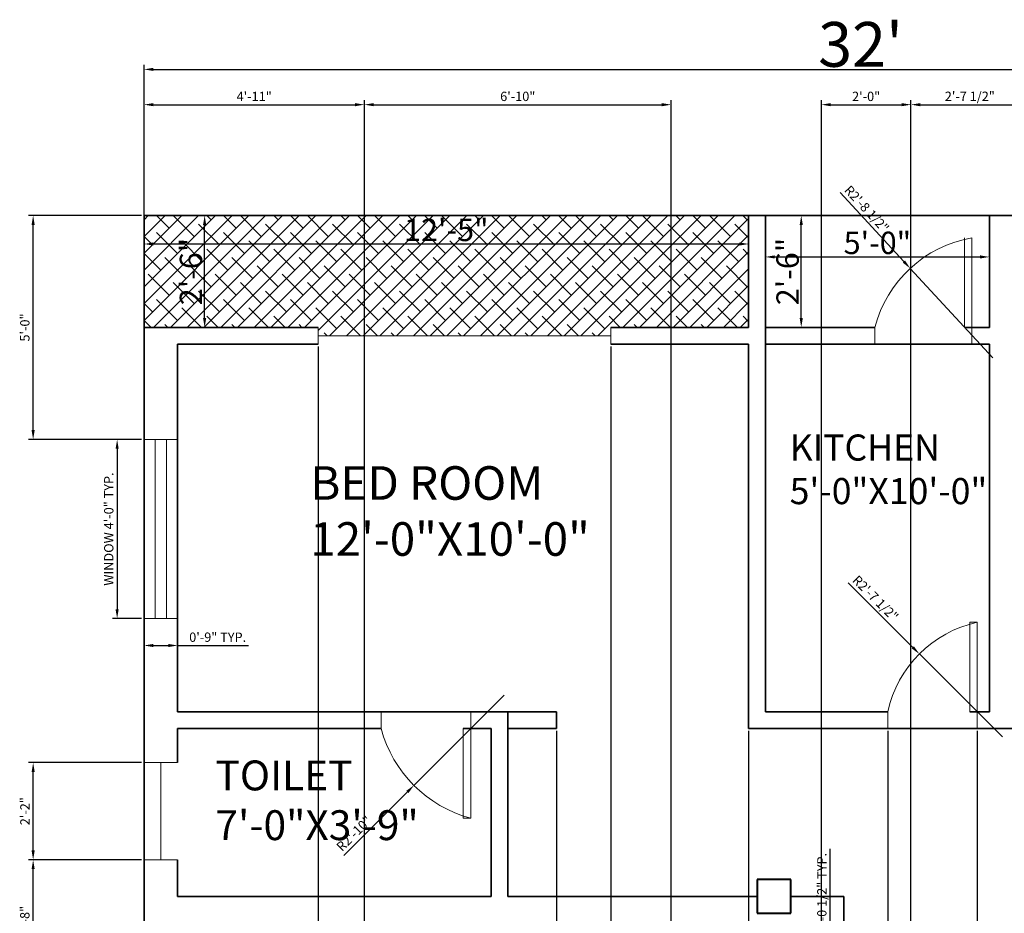
# Model space of a CAD drawing. Units: millimetres. Extents: x 2124 to 2653, y 1244 to 1836.
# Tile 3 of 4: x 2126 to 2390, y 1597 to 1836. Entities that reach past the tile are written whole.
import ezdxf

# ---------------------------------------------------------------- set-up
doc = ezdxf.new("R2010")
doc.units = ezdxf.units.MM
for name, color, linetype, lineweight in [('A-ANNO-DIMS', 2, 'Continuous', 18), ('A-AREA-IDEN', 7, 'Continuous', 18), ('A-COLS', 1, 'Continuous', 40), ('A-DOOR', 3, 'Continuous', 18), ('A-FLOR-PATT', 252, 'Continuous', 13), ('A-GLAZ', 4, 'Continuous', 18), ('A-WALL', 7, 'Continuous', 35)]:
    doc.layers.add(name, color=color, linetype=linetype, lineweight=lineweight)
doc.styles.get("Standard").update_dxf_attribs({"font": 'arial.ttf'})
doc.dimstyles.new('ISO-25', dxfattribs={"dimtxt": 2.5, "dimasz": 2.5, "dimexe": 1.25, "dimexo": 0.625, "dimtad": 1, "dimdec": 0, "dimlunit": 3, "dimtxsty": 'Standard', "dimcen": 2.5, "dimadec": 0, "dimazin": 0, "dimtfac": 1, "dimtdec": 0, "dimtmove": 0, "dimatfit": 3, "dimfxl": 1, "dimarcsym": 0})

# ---------------------------------------------------------------- blocks, each defined once
blk = doc.blocks.new('*D2')
at = {"layer": 'A-ANNO-DIMS', "color": 0, "lineweight": -2, "transparency": 16777216}
for p, q in [((2160.38, 1783.74), (2177.25, 1783.74)), ((2176, 1756.24), (2176, 1781.24)), ((2160.38, 1753.74), (2177.25, 1753.74))]:
    blk.add_line(p, q, dxfattribs=at)
at = {"layer": 'A-ANNO-DIMS', "color": 0, "transparency": 16777216}
for points in [[(2175.58, 1781.24), (2176.42, 1781.24), (2176, 1783.74)], [(2175.58, 1756.24), (2176.42, 1756.24), (2176, 1753.74)]]:
    blk.add_solid(points, dxfattribs=at)
at = {"layer": 'Defpoints', "color": 0, "transparency": 16777216}
for p in [(2159.76, 1783.74), (2176, 1783.74), (2159.76, 1753.74)]:
    blk.add_point(p, dxfattribs=at)
at = {"layer": 'A-ANNO-DIMS', "color": 0, "transparency": 16777216, "insert": (2172.34, 1768.74), "char_height": 2.5, "attachment_point": 5, "rotation": 90}
blk.add_mtext('{\\fCambria|b0|i0|c0|p18;\\H2.4x;2\'-6"}', dxfattribs=at)
blk = doc.blocks.new('*D3')
at = {"layer": 'A-ANNO-DIMS', "color": 0, "lineweight": -2, "transparency": 16777216}
for p, q in [((2326.88, 1783.74), (2337.1, 1783.74)), ((2335.85, 1756.24), (2335.85, 1781.24)), ((2326.88, 1753.74), (2337.1, 1753.74))]:
    blk.add_line(p, q, dxfattribs=at)
at = {"layer": 'A-ANNO-DIMS', "color": 0, "transparency": 16777216}
for points in [[(2335.44, 1781.24), (2336.27, 1781.24), (2335.85, 1783.74)], [(2335.44, 1756.24), (2336.27, 1756.24), (2335.85, 1753.74)]]:
    blk.add_solid(points, dxfattribs=at)
at = {"layer": 'Defpoints', "color": 0, "transparency": 16777216}
for p in [(2326.26, 1783.74), (2335.85, 1783.74), (2326.26, 1753.74)]:
    blk.add_point(p, dxfattribs=at)
at = {"layer": 'A-ANNO-DIMS', "color": 0, "transparency": 16777216, "insert": (2332.19, 1768.74), "char_height": 2.5, "width": 10.1505, "attachment_point": 5, "rotation": 90}
blk.add_mtext('{\\fCambria|b0|i0|c0|p18;\\H2.4x;2\'-6"}', dxfattribs=at)
blk = doc.blocks.new('*D4')
at = {"layer": 'A-ANNO-DIMS', "color": 0, "lineweight": -2, "transparency": 16777216}
for p, q in [((2326.26, 1783.12), (2326.26, 1771.39)), ((2386.26, 1783.12), (2386.26, 1771.39)), ((2328.76, 1772.64), (2383.76, 1772.64))]:
    blk.add_line(p, q, dxfattribs=at)
at = {"layer": 'A-ANNO-DIMS', "color": 0, "transparency": 16777216}
for points in [[(2328.76, 1773.06), (2328.76, 1772.22), (2326.26, 1772.64)], [(2383.76, 1773.06), (2383.76, 1772.22), (2386.26, 1772.64)]]:
    blk.add_solid(points, dxfattribs=at)
at = {"layer": 'Defpoints', "color": 0, "transparency": 16777216}
for p in [(2326.26, 1783.74), (2386.26, 1783.74), (2386.26, 1772.64)]:
    blk.add_point(p, dxfattribs=at)
at = {"layer": 'A-ANNO-DIMS', "color": 0, "transparency": 16777216, "insert": (2356.26, 1776.41), "char_height": 2.5, "width": 15.004, "attachment_point": 5}
blk.add_mtext('{\\fCambria|b0|i0|c0|p18;\\H2.4x;5\'-0"}', dxfattribs=at)
blk = doc.blocks.new('*D7')
at = {"layer": 'A-ANNO-DIMS', "color": 0, "lineweight": -2, "transparency": 16777216}
for p, q in [((2159.76, 1783.12), (2159.76, 1774.86)), ((2321.76, 1783.12), (2321.76, 1774.86)), ((2162.26, 1776.11), (2319.26, 1776.11))]:
    blk.add_line(p, q, dxfattribs=at)
at = {"layer": 'A-ANNO-DIMS', "color": 0, "transparency": 16777216}
for points in [[(2162.26, 1776.53), (2162.26, 1775.69), (2159.76, 1776.11)], [(2319.26, 1776.53), (2319.26, 1775.69), (2321.76, 1776.11)]]:
    blk.add_solid(points, dxfattribs=at)
at = {"layer": 'Defpoints', "color": 0, "transparency": 16777216}
for p in [(2159.76, 1783.74), (2321.76, 1783.74), (2321.76, 1776.11)]:
    blk.add_point(p, dxfattribs=at)
at = {"layer": 'A-ANNO-DIMS', "color": 0, "transparency": 16777216, "insert": (2240.76, 1779.88), "char_height": 2.5, "width": 11.5719, "attachment_point": 5}
blk.add_mtext('{\\fCambria|b0|i0|c0|p18;\\H2.4x;12\'-5"}', dxfattribs=at)
blk = doc.blocks.new('*D8')
at = {"layer": 'A-ANNO-DIMS', "color": 0, "lineweight": -2, "transparency": 16777216}
for p, q in [((2159.76, 1784.37), (2159.76, 1824.15)), ((2543.76, 1784.37), (2543.76, 1824.15)), ((2162.26, 1822.9), (2541.26, 1822.9))]:
    blk.add_line(p, q, dxfattribs=at)
at = {"layer": 'A-ANNO-DIMS', "color": 0, "transparency": 16777216}
for points in [[(2162.26, 1823.31), (2162.26, 1822.48), (2159.76, 1822.9)], [(2541.26, 1823.31), (2541.26, 1822.48), (2543.76, 1822.9)]]:
    blk.add_solid(points, dxfattribs=at)
at = {"layer": 'Defpoints', "color": 0, "transparency": 16777216}
for p in [(2543.76, 1822.9), (2159.76, 1783.74), (2543.76, 1783.74)]:
    blk.add_point(p, dxfattribs=at)
at = {"layer": 'A-ANNO-DIMS', "color": 0, "transparency": 16777216, "insert": (2351.76, 1829.59), "char_height": 2.5, "attachment_point": 5}
blk.add_mtext("{\\fCambria|b0|i0|c0|p18;\\H4.8x;32'}", dxfattribs=at)
blk = doc.blocks.new('WINDOW-4FT')
for p, q in [((48, 9), (0, 9)), ((0, 9), (0, 0)), ((48, 0), (48, 9)), ((48, 6), (0, 6)), ((48, 3), (0, 3)), ((0, 0), (48, 0))]:
    blk.add_line(p, q)
blk = doc.blocks.new('COLUMN-9IN-SQ')
for p, q in [((9, 9), (0, 9)), ((0, 9), (0, 0)), ((9, 0), (9, 9)), ((0, 0), (9, 0))]:
    blk.add_line(p, q)
blk = doc.blocks.new('*D14')
at = {"layer": 'A-ANNO-DIMS', "color": 0, "lineweight": -2, "transparency": 16777216}
for p, q in [((2159.13, 1723.72), (2151.31, 1723.72)), ((2152.56, 1721.22), (2152.56, 1678.22)), ((2159.13, 1675.72), (2151.31, 1675.72))]:
    blk.add_line(p, q, dxfattribs=at)
at = {"layer": 'A-ANNO-DIMS', "color": 0, "transparency": 16777216}
for points in [[(2152.14, 1721.22), (2152.97, 1721.22), (2152.56, 1723.72)], [(2152.14, 1678.22), (2152.97, 1678.22), (2152.56, 1675.72)]]:
    blk.add_solid(points, dxfattribs=at)
at = {"layer": 'Defpoints', "color": 0, "transparency": 16777216}
for p in [(2159.76, 1723.72), (2152.56, 1675.72), (2159.76, 1675.72)]:
    blk.add_point(p, dxfattribs=at)
at = {"layer": 'A-ANNO-DIMS', "color": 0, "transparency": 16777216, "insert": (2150.64, 1699.72), "char_height": 2.5, "attachment_point": 5, "rotation": 90}
blk.add_mtext('WINDOW 4\'-0" TYP.', dxfattribs=at)
blk = doc.blocks.new('*D15')
at = {"layer": 'A-ANNO-DIMS', "color": 0, "lineweight": -2, "transparency": 16777216}
for p, q in [((2159.76, 1675.1), (2159.76, 1667.27)), ((2168.76, 1675.1), (2168.76, 1667.27)), ((2162.26, 1668.52), (2166.26, 1668.52)), ((2168.76, 1668.52), (2187.75, 1668.52))]:
    blk.add_line(p, q, dxfattribs=at)
at = {"layer": 'A-ANNO-DIMS', "color": 0, "transparency": 16777216}
for points in [[(2162.26, 1668.94), (2162.26, 1668.1), (2159.76, 1668.52)], [(2166.26, 1668.94), (2166.26, 1668.1), (2168.76, 1668.52)]]:
    blk.add_solid(points, dxfattribs=at)
at = {"layer": 'Defpoints', "color": 0, "transparency": 16777216}
for p in [(2159.76, 1675.72), (2168.76, 1675.72), (2168.76, 1668.52)]:
    blk.add_point(p, dxfattribs=at)
at = {"layer": 'A-ANNO-DIMS', "color": 0, "transparency": 16777216, "insert": (2179.5, 1670.42), "char_height": 2.5, "attachment_point": 5}
blk.add_mtext('0\'-9" TYP.', dxfattribs=at)
blk = doc.blocks.new('*D20')
at = {"layer": 'A-ANNO-DIMS', "color": 0, "lineweight": -2, "transparency": 16777216}
for p, q in [((2343.62, 1579.62), (2343.62, 1614.03)), ((2346.63, 1579.62), (2342.37, 1579.62)), ((2343.62, 1557.86), (2343.62, 1577.12)), ((2346.63, 1555.36), (2342.37, 1555.36))]:
    blk.add_line(p, q, dxfattribs=at)
at = {"layer": 'A-ANNO-DIMS', "color": 0, "transparency": 16777216}
for points in [[(2343.2, 1577.12), (2344.04, 1577.12), (2343.62, 1579.62)], [(2343.2, 1557.86), (2344.04, 1557.86), (2343.62, 1555.36)]]:
    blk.add_solid(points, dxfattribs=at)
at = {"layer": 'Defpoints', "color": 0, "transparency": 16777216}
for p in [(2343.62, 1579.62), (2347.26, 1579.62), (2347.26, 1555.36)]:
    blk.add_point(p, dxfattribs=at)
at = {"layer": 'A-ANNO-DIMS', "color": 0, "transparency": 16777216, "insert": (2341.7, 1598.07), "char_height": 2.5, "attachment_point": 5, "rotation": 90}
blk.add_mtext('LEAF 2\'-0 1/2" TYP.', dxfattribs=at)
blk = doc.blocks.new('*D28')
at = {"layer": 'A-ANNO-DIMS', "color": 0, "lineweight": -2, "transparency": 16777216}
for p, q in [((2159.13, 1783.74), (2128.81, 1783.74)), ((2130.06, 1726.22), (2130.06, 1781.24)), ((2159.13, 1723.72), (2128.81, 1723.72))]:
    blk.add_line(p, q, dxfattribs=at)
at = {"layer": 'A-ANNO-DIMS', "color": 0, "transparency": 16777216}
for points in [[(2129.64, 1781.24), (2130.47, 1781.24), (2130.06, 1783.74)], [(2129.64, 1726.22), (2130.47, 1726.22), (2130.06, 1723.72)]]:
    blk.add_solid(points, dxfattribs=at)
at = {"layer": 'Defpoints', "color": 0, "transparency": 16777216}
for p in [(2130.06, 1783.74), (2159.76, 1783.74), (2159.76, 1723.72)]:
    blk.add_point(p, dxfattribs=at)
at = {"layer": 'A-ANNO-DIMS', "color": 0, "transparency": 16777216, "insert": (2128.15, 1753.73), "char_height": 2.5, "attachment_point": 5, "rotation": 90}
blk.add_mtext('5\'-0"', dxfattribs=at)
blk = doc.blocks.new('*D34')
at = {"layer": 'A-ANNO-DIMS', "color": 0, "lineweight": -2, "transparency": 16777216}
for p, q in [((2159.13, 1611.09), (2128.81, 1611.09)), ((2130.06, 1581.36), (2130.06, 1608.59)), ((2159.13, 1578.86), (2128.81, 1578.86))]:
    blk.add_line(p, q, dxfattribs=at)
at = {"layer": 'A-ANNO-DIMS', "color": 0, "transparency": 16777216}
for points in [[(2129.64, 1608.59), (2130.47, 1608.59), (2130.06, 1611.09)], [(2129.64, 1581.36), (2130.47, 1581.36), (2130.06, 1578.86)]]:
    blk.add_solid(points, dxfattribs=at)
at = {"layer": 'Defpoints', "color": 0, "transparency": 16777216}
for p in [(2130.06, 1611.09), (2159.76, 1611.09), (2159.76, 1578.86)]:
    blk.add_point(p, dxfattribs=at)
at = {"layer": 'A-ANNO-DIMS', "color": 0, "transparency": 16777216, "insert": (2128.15, 1594.98), "char_height": 2.5, "attachment_point": 5, "rotation": 90}
blk.add_mtext('2\'-8"', dxfattribs=at)
blk = doc.blocks.new('*D35')
at = {"layer": 'A-ANNO-DIMS', "color": 0, "lineweight": -2, "transparency": 16777216}
for p, q in [((2159.13, 1637.13), (2128.81, 1637.13)), ((2130.06, 1613.59), (2130.06, 1634.63)), ((2159.13, 1611.09), (2128.81, 1611.09))]:
    blk.add_line(p, q, dxfattribs=at)
at = {"layer": 'A-ANNO-DIMS', "color": 0, "transparency": 16777216}
for points in [[(2129.64, 1634.63), (2130.47, 1634.63), (2130.06, 1637.13)], [(2129.64, 1613.59), (2130.47, 1613.59), (2130.06, 1611.09)]]:
    blk.add_solid(points, dxfattribs=at)
at = {"layer": 'Defpoints', "color": 0, "transparency": 16777216}
for p in [(2130.06, 1637.13), (2159.76, 1637.13), (2159.76, 1611.09)]:
    blk.add_point(p, dxfattribs=at)
at = {"layer": 'A-ANNO-DIMS', "color": 0, "transparency": 16777216, "insert": (2128.18, 1624.11), "char_height": 2.5, "attachment_point": 5, "rotation": 90}
blk.add_mtext('2\'-2"', dxfattribs=at)
blk = doc.blocks.new('*D36')
at = {"layer": 'A-ANNO-DIMS', "color": 0, "lineweight": -2, "transparency": 16777216}
for p, q in [((2159.76, 1753.12), (2159.76, 1256.02)), ((2206.41, 1748.62), (2206.41, 1256.02)), ((2162.26, 1257.27), (2203.91, 1257.27))]:
    blk.add_line(p, q, dxfattribs=at)
at = {"layer": 'A-ANNO-DIMS', "color": 0, "transparency": 16777216}
for points in [[(2162.26, 1257.69), (2162.26, 1256.86), (2159.76, 1257.27)], [(2203.91, 1257.69), (2203.91, 1256.86), (2206.41, 1257.27)]]:
    blk.add_solid(points, dxfattribs=at)
at = {"layer": 'Defpoints', "color": 0, "transparency": 16777216}
for p in [(2159.76, 1753.74), (2206.41, 1749.24), (2206.41, 1257.27)]:
    blk.add_point(p, dxfattribs=at)
at = {"layer": 'A-ANNO-DIMS', "color": 0, "transparency": 16777216, "insert": (2183.08, 1259.19), "char_height": 2.5, "attachment_point": 5}
blk.add_mtext('3\'-10 1/2"', dxfattribs=at)
blk = doc.blocks.new('*D37')
at = {"layer": 'A-ANNO-DIMS', "color": 0, "lineweight": -2, "transparency": 16777216}
for p, q in [((2206.41, 1748.62), (2206.41, 1256.02)), ((2284.8, 1748.62), (2284.8, 1256.02)), ((2208.91, 1257.27), (2282.3, 1257.27))]:
    blk.add_line(p, q, dxfattribs=at)
at = {"layer": 'A-ANNO-DIMS', "color": 0, "transparency": 16777216}
for points in [[(2208.91, 1257.69), (2208.91, 1256.86), (2206.41, 1257.27)], [(2282.3, 1257.69), (2282.3, 1256.86), (2284.8, 1257.27)]]:
    blk.add_solid(points, dxfattribs=at)
at = {"layer": 'Defpoints', "color": 0, "transparency": 16777216}
for p in [(2206.41, 1749.24), (2284.8, 1749.24), (2284.8, 1257.27)]:
    blk.add_point(p, dxfattribs=at)
at = {"layer": 'A-ANNO-DIMS', "color": 0, "transparency": 16777216, "insert": (2245.61, 1259.19), "char_height": 2.5, "attachment_point": 5}
blk.add_mtext('6\'-6 1/2"', dxfattribs=at)
blk = doc.blocks.new('*D38')
at = {"layer": 'A-ANNO-DIMS', "color": 0, "lineweight": -2, "transparency": 16777216}
for p, q in [((2159.76, 1319.87), (2159.76, 1814.69)), ((2162.26, 1813.44), (2216.31, 1813.44)), ((2218.81, 1324.37), (2218.81, 1814.69))]:
    blk.add_line(p, q, dxfattribs=at)
at = {"layer": 'A-ANNO-DIMS', "color": 0, "transparency": 16777216}
for points in [[(2162.26, 1813.86), (2162.26, 1813.02), (2159.76, 1813.44)], [(2216.31, 1813.86), (2216.31, 1813.02), (2218.81, 1813.44)]]:
    blk.add_solid(points, dxfattribs=at)
at = {"layer": 'Defpoints', "color": 0, "transparency": 16777216}
for p in [(2218.81, 1813.44), (2218.81, 1323.74), (2159.76, 1319.24)]:
    blk.add_point(p, dxfattribs=at)
at = {"layer": 'A-ANNO-DIMS', "color": 0, "transparency": 16777216, "insert": (2189.28, 1815.32), "char_height": 2.5, "attachment_point": 5}
blk.add_mtext('4\'-11"', dxfattribs=at)
blk = doc.blocks.new('*D39')
at = {"layer": 'A-ANNO-DIMS', "color": 0, "lineweight": -2, "transparency": 16777216}
for p, q in [((2218.81, 1324.37), (2218.81, 1814.69)), ((2221.31, 1813.44), (2298.49, 1813.44)), ((2300.99, 1324.37), (2300.99, 1814.69))]:
    blk.add_line(p, q, dxfattribs=at)
at = {"layer": 'A-ANNO-DIMS', "color": 0, "transparency": 16777216}
for points in [[(2221.31, 1813.86), (2221.31, 1813.02), (2218.81, 1813.44)], [(2298.49, 1813.86), (2298.49, 1813.02), (2300.99, 1813.44)]]:
    blk.add_solid(points, dxfattribs=at)
at = {"layer": 'Defpoints', "color": 0, "transparency": 16777216}
for p in [(2300.99, 1813.44), (2218.81, 1323.74), (2300.99, 1323.74)]:
    blk.add_point(p, dxfattribs=at)
at = {"layer": 'A-ANNO-DIMS', "color": 0, "transparency": 16777216, "insert": (2259.9, 1815.34), "char_height": 2.5, "attachment_point": 5}
blk.add_mtext('6\'-10"', dxfattribs=at)
blk = doc.blocks.new('*D40')
at = {"layer": 'A-ANNO-DIMS', "color": 0, "lineweight": -2, "transparency": 16777216}
for p, q in [((2270.27, 1645.62), (2270.27, 1256.02)), ((2321.76, 1645.62), (2321.76, 1256.02)), ((2272.77, 1257.27), (2319.26, 1257.27))]:
    blk.add_line(p, q, dxfattribs=at)
at = {"layer": 'A-ANNO-DIMS', "color": 0, "transparency": 16777216}
for points in [[(2272.77, 1257.69), (2272.77, 1256.86), (2270.27, 1257.27)], [(2319.26, 1257.69), (2319.26, 1256.86), (2321.76, 1257.27)]]:
    blk.add_solid(points, dxfattribs=at)
at = {"layer": 'Defpoints', "color": 0, "transparency": 16777216}
for p in [(2270.27, 1646.24), (2321.76, 1646.24), (2321.76, 1257.27)]:
    blk.add_point(p, dxfattribs=at)
at = {"layer": 'A-ANNO-DIMS', "color": 0, "transparency": 16777216, "insert": (2296.01, 1259.19), "char_height": 2.5, "attachment_point": 5}
blk.add_mtext('4\'-3 1/2"', dxfattribs=at)
blk = doc.blocks.new('*D41')
at = {"layer": 'A-ANNO-DIMS', "color": 0, "lineweight": -2, "transparency": 16777216}
for p, q in [((2321.76, 1645.62), (2321.76, 1256.02)), ((2359.02, 1645.62), (2359.02, 1256.02)), ((2324.26, 1257.27), (2356.52, 1257.27))]:
    blk.add_line(p, q, dxfattribs=at)
at = {"layer": 'A-ANNO-DIMS', "color": 0, "transparency": 16777216}
for points in [[(2324.26, 1257.69), (2324.26, 1256.86), (2321.76, 1257.27)], [(2356.52, 1257.69), (2356.52, 1256.86), (2359.02, 1257.27)]]:
    blk.add_solid(points, dxfattribs=at)
at = {"layer": 'Defpoints', "color": 0, "transparency": 16777216}
for p in [(2321.76, 1646.24), (2359.02, 1646.24), (2359.02, 1257.27)]:
    blk.add_point(p, dxfattribs=at)
at = {"layer": 'A-ANNO-DIMS', "color": 0, "transparency": 16777216, "insert": (2340.39, 1259.19), "char_height": 2.5, "attachment_point": 5}
blk.add_mtext('3\'-1 1/2"', dxfattribs=at)
blk = doc.blocks.new('*D42')
at = {"layer": 'A-ANNO-DIMS', "color": 0, "lineweight": -2, "transparency": 16777216}
for p, q in [((2359.02, 1645.62), (2359.02, 1256.02)), ((2383.02, 1645.62), (2383.02, 1256.02)), ((2361.52, 1257.27), (2380.52, 1257.27))]:
    blk.add_line(p, q, dxfattribs=at)
at = {"layer": 'A-ANNO-DIMS', "color": 0, "transparency": 16777216}
for points in [[(2361.52, 1257.69), (2361.52, 1256.86), (2359.02, 1257.27)], [(2380.52, 1257.69), (2380.52, 1256.86), (2383.02, 1257.27)]]:
    blk.add_solid(points, dxfattribs=at)
at = {"layer": 'Defpoints', "color": 0, "transparency": 16777216}
for p in [(2359.02, 1646.24), (2383.02, 1646.24), (2383.02, 1257.27)]:
    blk.add_point(p, dxfattribs=at)
at = {"layer": 'A-ANNO-DIMS', "color": 0, "transparency": 16777216, "insert": (2371.02, 1259.18), "char_height": 2.5, "attachment_point": 5}
blk.add_mtext('2\'-0"', dxfattribs=at)
blk = doc.blocks.new('*D43')
at = {"layer": 'A-ANNO-DIMS', "color": 0, "lineweight": -2, "transparency": 16777216}
for p, q in [((2383.02, 1645.62), (2383.02, 1256.02)), ((2394.21, 1645.62), (2394.21, 1256.02)), ((2385.52, 1257.27), (2391.71, 1257.27))]:
    blk.add_line(p, q, dxfattribs=at)
at = {"layer": 'A-ANNO-DIMS', "color": 0, "transparency": 16777216}
for points in [[(2385.52, 1257.69), (2385.52, 1256.86), (2383.02, 1257.27)], [(2391.71, 1257.69), (2391.71, 1256.86), (2394.21, 1257.27)]]:
    blk.add_solid(points, dxfattribs=at)
at = {"layer": 'Defpoints', "color": 0, "transparency": 16777216}
for p in [(2383.02, 1646.24), (2394.21, 1646.24), (2394.21, 1257.27)]:
    blk.add_point(p, dxfattribs=at)
at = {"layer": 'A-ANNO-DIMS', "color": 0, "transparency": 16777216, "insert": (2388.62, 1259.18), "char_height": 2.5, "attachment_point": 5}
blk.add_mtext('0\'-11"', dxfattribs=at)
blk = doc.blocks.new('*D46')
at = {"layer": 'A-ANNO-DIMS', "color": 0, "lineweight": -2, "transparency": 16777216}
for p, q in [((2341.24, 1448.87), (2341.24, 1814.69)), ((2343.74, 1813.44), (2362.74, 1813.44)), ((2365.24, 1448.87), (2365.24, 1814.69))]:
    blk.add_line(p, q, dxfattribs=at)
at = {"layer": 'A-ANNO-DIMS', "color": 0, "transparency": 16777216}
for points in [[(2343.74, 1813.86), (2343.74, 1813.02), (2341.24, 1813.44)], [(2362.74, 1813.86), (2362.74, 1813.02), (2365.24, 1813.44)]]:
    blk.add_solid(points, dxfattribs=at)
at = {"layer": 'Defpoints', "color": 0, "transparency": 16777216}
for p in [(2365.24, 1813.44), (2341.24, 1448.24), (2365.24, 1448.24)]:
    blk.add_point(p, dxfattribs=at)
at = {"layer": 'A-ANNO-DIMS', "color": 0, "transparency": 16777216, "insert": (2353.24, 1815.34), "char_height": 2.5, "attachment_point": 5}
blk.add_mtext('2\'-0"', dxfattribs=at)
blk = doc.blocks.new('*D47')
at = {"layer": 'A-ANNO-DIMS', "color": 0, "lineweight": -2, "transparency": 16777216}
for p, q in [((2365.24, 1448.87), (2365.24, 1814.69)), ((2367.74, 1813.44), (2394.29, 1813.44)), ((2396.79, 1448.87), (2396.79, 1814.69))]:
    blk.add_line(p, q, dxfattribs=at)
at = {"layer": 'A-ANNO-DIMS', "color": 0, "transparency": 16777216}
for points in [[(2367.74, 1813.86), (2367.74, 1813.02), (2365.24, 1813.44)], [(2394.29, 1813.86), (2394.29, 1813.02), (2396.79, 1813.44)]]:
    blk.add_solid(points, dxfattribs=at)
at = {"layer": 'Defpoints', "color": 0, "transparency": 16777216}
for p in [(2396.79, 1813.44), (2365.24, 1448.24), (2396.79, 1448.24)]:
    blk.add_point(p, dxfattribs=at)
at = {"layer": 'A-ANNO-DIMS', "color": 0, "transparency": 16777216, "insert": (2381.02, 1815.36), "char_height": 2.5, "attachment_point": 5}
blk.add_mtext('2\'-7 1/2"', dxfattribs=at)
blk = doc.blocks.new('*D55')
at = {"layer": 'A-ANNO-DIMS', "color": 0, "lineweight": -2, "transparency": 16777216}
for p, q in [((2256.25, 1655.2), (2232.1, 1631.05)), ((2213.28, 1612.23), (2230.33, 1629.28))]:
    blk.add_line(p, q, dxfattribs=at)
at = {"layer": 'A-ANNO-DIMS', "color": 0, "transparency": 16777216}
blk.add_solid([(2230.03, 1629.58), (2230.62, 1628.99), (2232.1, 1631.05)], dxfattribs=at)
at = {"layer": 'Defpoints', "color": 0, "transparency": 16777216}
for p in [(2256.25, 1655.2), (2232.1, 1631.05)]:
    blk.add_point(p, dxfattribs=at)
at = {"layer": 'A-ANNO-DIMS', "color": 0, "transparency": 16777216, "insert": (2216.26, 1617.9), "char_height": 2.5, "attachment_point": 5, "rotation": 44.9997}
blk.add_mtext('R2\'-10"', dxfattribs=at)
blk = doc.blocks.new('*D56')
at = {"layer": 'A-ANNO-DIMS', "color": 0, "lineweight": -2, "transparency": 16777216}
for p, q in [((2346.29, 1789.89), (2363.36, 1771.4)), ((2387.21, 1745.56), (2365.05, 1769.57))]:
    blk.add_line(p, q, dxfattribs=at)
at = {"layer": 'A-ANNO-DIMS', "color": 0, "transparency": 16777216}
blk.add_solid([(2363.66, 1771.68), (2363.05, 1771.12), (2365.05, 1769.57)], dxfattribs=at)
at = {"layer": 'Defpoints', "color": 0, "transparency": 16777216}
for p in [(2365.05, 1769.57), (2387.21, 1745.56)]:
    blk.add_point(p, dxfattribs=at)
at = {"layer": 'A-ANNO-DIMS', "color": 0, "transparency": 16777216, "insert": (2353.16, 1785.27), "char_height": 2.5, "attachment_point": 5, "rotation": 312.7096}
blk.add_mtext('R2\'-8 1/2"', dxfattribs=at)
blk = doc.blocks.new('*D58')
at = {"layer": 'A-ANNO-DIMS', "color": 0, "lineweight": -2, "transparency": 16777216}
for p, q in [((2348.46, 1685.3), (2365.74, 1668.02)), ((2389.77, 1644), (2367.51, 1666.25))]:
    blk.add_line(p, q, dxfattribs=at)
at = {"layer": 'A-ANNO-DIMS', "color": 0, "transparency": 16777216}
blk.add_solid([(2366.04, 1668.31), (2365.45, 1667.73), (2367.51, 1666.25)], dxfattribs=at)
at = {"layer": 'Defpoints', "color": 0, "transparency": 16777216}
for p in [(2367.51, 1666.25), (2389.77, 1644)]:
    blk.add_point(p, dxfattribs=at)
at = {"layer": 'A-ANNO-DIMS', "color": 0, "transparency": 16777216, "insert": (2355.51, 1680.96), "char_height": 2.5, "attachment_point": 5, "rotation": 315}
blk.add_mtext('R2\'-7 1/2"', dxfattribs=at)

msp = doc.modelspace()

# ---------------------------------------------------------------- hatches: boundary and pattern name
at = {"layer": 'A-FLOR-PATT'}
h = msp.add_hatch(dxfattribs=at)
h.set_pattern_fill('ANSI38', color=256)
h.paths.add_polyline_path([(2321.76, 1783.74), (2159.76, 1783.74), (2159.76, 1753.74), (2206.41, 1753.74), (2206.41, 1751.49), (2284.8, 1751.49), (2284.8, 1753.74), (2321.76, 1753.74)])
h.paths.add_polyline_path([(2300.96, 1321.49), (2218.81, 1321.49), (2218.81, 1319.24), (2159.76, 1319.24), (2159.76, 1286.97), (2341.76, 1286.97), (2341.76, 1319.24), (2337.34, 1319.24), (2337.34, 1295.24, -0.529331)])
h.paths.add_polyline_path([(2169.36, 1293.27), (2169.36, 1312.93), (2157.68, 1312.93), (2157.68, 1293.27)], flags=9)
h.paths.add_polyline_path([(2232.46, 1289.84), (2268.72, 1289.84), (2268.72, 1306.74), (2232.46, 1306.74)], flags=24)

# ---------------------------------------------------------------- linework, layer by layer
at = {"layer": 'A-DOOR'}
for p, q in [((2379.58, 1777.74), (2379.58, 1753.74)), ((2381.58, 1753.74), (2381.58, 1777.74)), ((2355.58, 1753.74), (2355.58, 1749.24)), ((2381.58, 1753.74), (2381.58, 1749.24)), ((2383.02, 1674.74), (2381.02, 1674.74)), ((2381.02, 1674.74), (2381.02, 1650.74)), ((2383.02, 1650.74), (2383.02, 1674.74)), ((2223.29, 1650.74), (2223.29, 1646.24)), ((2247.29, 1650.74), (2247.29, 1646.24)), ((2359.02, 1650.74), (2359.02, 1646.24)), ((2383.02, 1650.74), (2383.02, 1646.24)), ((2245.29, 1622.24), (2245.29, 1646.24)), ((2247.29, 1646.24), (2247.29, 1622.24)), ((2247.29, 1622.24), (2245.29, 1622.24))]:
    msp.add_line(p, q, dxfattribs=at)
for centre, radius, start, end in [((2387.21, 1745.56), 32.67, 99.92, 165.4988), ((2389.77, 1644), 31.48, 102.3741, 167.6259), ((2256.25, 1655.2), 34.16, 195.2123, 254.7877)]:
    msp.add_arc(centre, radius, start, end, dxfattribs=at)
at = {"layer": 'A-GLAZ'}
for p, q in [((2206.41, 1753.74), (2206.41, 1749.24)), ((2284.8, 1753.74), (2284.8, 1749.24)), ((2206.41, 1751.49), (2284.95, 1751.49)), ((2159.76, 1637.13), (2168.76, 1637.13)), ((2164.26, 1637.13), (2164.26, 1611.09)), ((2159.76, 1611.09), (2168.76, 1611.09))]:
    msp.add_line(p, q, dxfattribs=at)
at = {"layer": 'A-WALL'}
for p, q in [((2543.76, 1783.74), (2159.76, 1783.74)), ((2159.76, 1783.74), (2159.76, 1637.13)), ((2321.76, 1753.74), (2321.76, 1783.74)), ((2326.26, 1650.74), (2326.26, 1783.74)), ((2386.26, 1753.74), (2386.26, 1783.74)), ((2206.41, 1753.74), (2159.76, 1753.74)), ((2321.76, 1753.74), (2284.8, 1753.74)), ((2355.58, 1753.74), (2326.26, 1753.74)), ((2386.26, 1753.74), (2379.58, 1753.74)), ((2168.76, 1749.24), (2168.76, 1650.74)), ((2206.41, 1749.24), (2168.76, 1749.24)), ((2321.76, 1749.24), (2284.8, 1749.24)), ((2321.76, 1646.24), (2321.76, 1749.24)), ((2386.26, 1749.24), (2326.26, 1749.24)), ((2386.26, 1650.74), (2386.26, 1749.24)), ((2270.27, 1650.74), (2168.76, 1650.74)), ((2257.26, 1650.74), (2257.26, 1601.24)), ((2270.27, 1646.24), (2270.27, 1650.74)), ((2359.02, 1650.74), (2326.26, 1650.74)), ((2386.26, 1650.74), (2381.02, 1650.74)), ((2223.29, 1646.24), (2168.76, 1646.24)), ((2168.76, 1646.24), (2168.76, 1637.13)), ((2252.76, 1646.24), (2245.29, 1646.24)), ((2252.76, 1646.24), (2252.76, 1601.24)), ((2270.27, 1646.24), (2257.26, 1646.24)), ((2386.26, 1646.24), (2321.76, 1646.24)), ((2534.76, 1646.24), (2383.02, 1646.24)), ((2159.76, 1611.09), (2159.76, 1578.86)), ((2168.76, 1611.09), (2168.76, 1601.24)), ((2252.76, 1601.24), (2168.76, 1601.24)), ((2324.08, 1601.24), (2257.26, 1601.24)), ((2347.26, 1601.24), (2333.08, 1601.24)), ((2347.26, 1601.24), (2347.26, 1579.36))]:
    msp.add_line(p, q, dxfattribs=at)

# ---------------------------------------------------------------- block references
at = {"layer": 'A-COLS'}
msp.add_blockref('COLUMN-9IN-SQ', (2324.08, 1596.77), dxfattribs=at)
at = {"layer": 'A-GLAZ', "rotation": 270.0000000000009}
msp.add_blockref('WINDOW-4FT', (2159.76, 1723.72), dxfattribs=at)

# ---------------------------------------------------------------- texts
at = {"layer": 'A-AREA-IDEN', "attachment_point": 1}
for s, width, insert, char_height in [('{\\fCambria|b0|i0|c0|p18;KITCHEN\\P5\'-0"X10\'-0"}', 49.1713, (2332.75, 1725.06), 7), ('{\\fCambria|b0|i0|c0|p18;BED ROOM\\P12\'-0"X10\'-0"}', 93.0425, (2204.3, 1716.56), 9), ('{\\fCambria|b0|i0|c0|p18;TOILET\\P7\'-0"X3\'-9"}', 45.7785, (2178.9, 1637.7), 8)]:
    msp.add_mtext_dynamic_manual_height_columns(s, width=width, gutter_width=12.5, heights=[0], dxfattribs=dict(at, insert=insert, char_height=char_height))

# ---------------------------------------------------------------- dimensions: what is measured, and where the dimension line sits
at = {"layer": 'A-ANNO-DIMS'}
for base, p2, text, picture, middle in [((2543.76, 1822.9), (2543.76, 1783.74), '{\\fCambria|b0|i0|c0|p18;\\H4.8x;<>}', '*D8', (2351.76, 1829.59)), ((2321.76, 1776.11), (2321.76, 1783.74), '{\\fCambria|b0|i0|c0|p18;\\H2.4x;12\'-5"}', '*D7', (2240.76, 1779.88))]:
    dim = msp.add_linear_dim(base=base, p1=(2159.76, 1783.74), p2=p2, text=text, dimstyle='ISO-25', override={"dimclrd": 0, "dimclre": 0, "dimclrt": 0}, dxfattribs=at)
    dim.commit()
    dim.dimension.update_dxf_attribs({"geometry": picture, "text_midpoint": middle})
for base, p1, p2, picture, middle in [((2396.7929, 1813.4406), (2365.2427, 1448.2406), (2396.7929, 1448.2406), '*D47', (2381.0178, 1815.3582)), ((2218.8056, 1813.4406), (2159.7564, 1319.2406), (2218.8056, 1323.7406), '*D38', (2189.281, 1815.3207)), ((2300.99, 1813.44), (2218.81, 1323.74), (2300.99, 1323.74), '*D39', (2259.9, 1815.34)), ((2365.24, 1813.44), (2341.24, 1448.24), (2365.24, 1448.24), '*D46', (2353.24, 1815.34)), ((2206.4099, 1257.2741), (2159.7564, 1753.7406), (2206.4099, 1749.2406), '*D36', (2183.0831, 1259.1926)), ((2284.8, 1257.27), (2206.41, 1749.24), (2284.8, 1749.24), '*D37', (2245.61, 1259.19)), ((2321.76, 1257.27), (2270.27, 1646.24), (2321.76, 1646.24), '*D40', (2296.01, 1259.19)), ((2359.02, 1257.27), (2321.76, 1646.24), (2359.02, 1646.24), '*D41', (2340.39, 1259.19)), ((2383.02, 1257.27), (2359.02, 1646.24), (2383.02, 1646.24), '*D42', (2371.02, 1259.18)), ((2394.21, 1257.27), (2383.02, 1646.24), (2394.21, 1646.24), '*D43', (2388.62, 1259.18))]:
    dim = msp.add_linear_dim(base=base, p1=p1, p2=p2, dimstyle='ISO-25', override={"dimdec": 1, "dimlfac": 1, "dimrnd": 0, "dimzin": 1, "dimdsep": 46, "dimlunit": 4, "dimfrac": 2}, dxfattribs=at)
    dim.commit()
    dim.dimension.update_dxf_attribs({"geometry": picture, "text_midpoint": middle})
for center, mpoint, picture, middle in [((2387.21, 1745.56), (2365.05, 1769.57), '*D56', (2351.76, 1783.97)), ((2389.77, 1644), (2367.51, 1666.25), '*D58', (2354.16, 1679.61)), ((2256.25, 1655.2), (2232.1, 1631.05), '*D55', (2217.6, 1616.56))]:
    dim = msp.add_radius_dim(center=center, mpoint=mpoint, dimstyle='ISO-25', override={"dimdec": 1, "dimlfac": 1, "dimrnd": 0, "dimzin": 1, "dimdsep": 46, "dimlunit": 4, "dimfrac": 2}, dxfattribs=at)
    dim.commit()
    dim.dimension.update_dxf_attribs({"geometry": picture, "text_midpoint": middle, "dimtype": 164})
for base, p1, p2, picture, middle in [((2130.06, 1783.74), (2159.76, 1723.72), (2159.76, 1783.74), '*D28', (2128.15, 1753.73)), ((2130.06, 1637.13), (2159.76, 1611.09), (2159.76, 1637.13), '*D35', (2128.18, 1624.11)), ((2130.06, 1611.09), (2159.76, 1578.86), (2159.76, 1611.09), '*D34', (2128.15, 1594.98))]:
    dim = msp.add_linear_dim(base=base, p1=p1, p2=p2, angle=90, dimstyle='ISO-25', override={"dimdec": 1, "dimlfac": 1, "dimrnd": 0, "dimzin": 1, "dimdsep": 46, "dimlunit": 4, "dimfrac": 2}, dxfattribs=at)
    dim.commit()
    dim.dimension.update_dxf_attribs({"geometry": picture, "text_midpoint": middle})
for base, p1, p2, angle, text, override, picture, middle in [((2176, 1783.74), (2159.76, 1753.74), (2159.76, 1783.74), 90, '{\\fCambria|b0|i0|c0|p18;\\H2.4x;<>}', {"dimclrd": 0, "dimclre": 0, "dimclrt": 0}, '*D2', (2172.34, 1768.74)), ((2335.85, 1783.74), (2326.26, 1753.74), (2326.26, 1783.74), 90, '{\\fCambria|b0|i0|c0|p18;\\H2.4x;2\'-6"}', {"dimclrd": 0, "dimclre": 0, "dimclrt": 0}, '*D3', (2332.19, 1768.74)), ((2152.56, 1675.72), (2159.76, 1723.72), (2159.76, 1675.72), 270, 'WINDOW <> TYP.', {"dimdec": 1, "dimlfac": 1, "dimrnd": 0, "dimzin": 1, "dimdsep": 46, "dimlunit": 4, "dimfrac": 2}, '*D14', (2150.64, 1699.72)), ((2168.76, 1668.52), (2159.76, 1675.72), (2168.76, 1675.72), 0, '<> TYP.', {"dimdec": 1, "dimlfac": 1, "dimrnd": 0, "dimzin": 1, "dimdsep": 46, "dimlunit": 4, "dimfrac": 2}, '*D15', (2179.5, 1670.42)), ((2343.62, 1579.62), (2347.26, 1555.36), (2347.26, 1579.62), 90, 'LEAF <> TYP.', {"dimdec": 1, "dimlfac": 1, "dimrnd": 0, "dimzin": 1, "dimdsep": 46, "dimlunit": 4, "dimfrac": 2}, '*D20', (2341.7, 1598.07))]:
    dim = msp.add_linear_dim(base=base, p1=p1, p2=p2, angle=angle, text=text, dimstyle='ISO-25', override=override, dxfattribs=at)
    dim.commit()
    dim.dimension.update_dxf_attribs({"geometry": picture, "text_midpoint": middle})
dim = msp.add_linear_dim(base=(2386.26, 1772.64), p1=(2326.26, 1783.74), p2=(2386.26, 1783.74), text='{\\fCambria|b0|i0|c0|p18;\\H2.4x;5\'-0"}', dimstyle='ISO-25', override={"dimclrd": 0, "dimclre": 0, "dimclrt": 0}, dxfattribs=at)
dim.commit()
dim.dimension.update_dxf_attribs({"geometry": '*D4', "text_midpoint": (2356.26, 1772.64), "dimtype": 160})

doc.saveas('drawing.dxf')
